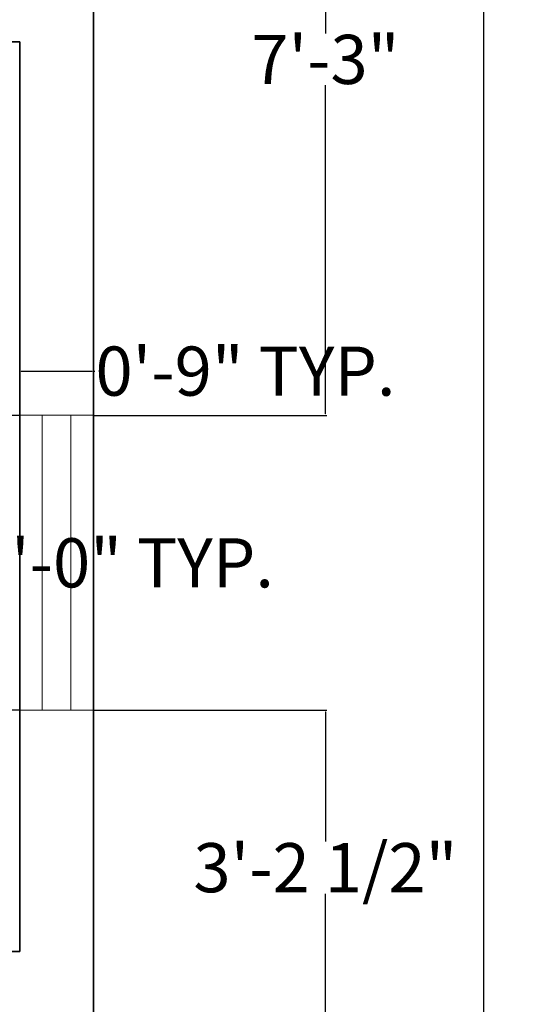
# Model space of a CAD drawing. Units: inches. Extents: x -26 to 575, y -18 to 513.
# Tile 18 of 28: x 513 to 575, y 121 to 241. Entities that reach past the tile are written whole.
import ezdxf

# ---------------------------------------------------------------- set-up
doc = ezdxf.new("R2010")
doc.units = ezdxf.units.IN
doc.header["$MEASUREMENT"] = 0
for name, color, linetype, lineweight in [('A-ANNO-DIMS', 2, 'Continuous', 18), ('A-GLAZ', 4, 'Continuous', 18), ('A-WALL', 7, 'Continuous', 35)]:
    doc.layers.add(name, color=color, linetype=linetype, lineweight=lineweight)
doc.styles.get("Standard").update_dxf_attribs({"font": 'arial.ttf', "height": 6})
doc.dimstyles.get("Standard").update_dxf_attribs({"dimtxt": 6, "dimasz": 0.18, "dimexe": 0.18, "dimexo": 0.0625, "dimgap": 0.09, "dimtad": 0, "dimtih": 1, "dimtoh": 1, "dimzin": 0, "dimdsep": 46, "dimlunit": 3, "dimtxsty": 'Standard', "dimcen": 0.09, "dimadec": 0, "dimazin": 0, "dimtfac": 1, "dimtofl": 0, "dimtmove": 0, "dimatfit": 3, "dimfxl": 1, "dimtolj": 1, "dimtzin": 0, "dimarcsym": 0})

# ---------------------------------------------------------------- blocks, each defined once
blk = doc.blocks.new('*D2')
at = {"layer": 'A-ANNO-DIMS', "color": 0, "lineweight": -2, "transparency": 16777216}
for p, q in [((522.24, 475.51), (569.98, 475.51)), ((569.8, 475.33), (569.8, 250.66)), ((569.8, 19.69), (569.8, 244.35)), ((522.24, 19.51), (569.98, 19.51))]:
    blk.add_line(p, q, dxfattribs=at)
at = {"layer": 'A-ANNO-DIMS', "color": 0, "transparency": 16777216}
for points in [[(569.77, 475.33), (569.83, 475.33), (569.8, 475.51)], [(569.77, 19.69), (569.83, 19.69), (569.8, 19.51)]]:
    blk.add_solid(points, dxfattribs=at)
at = {"layer": 'Defpoints', "color": 0, "transparency": 16777216}
for p in [(522.18, 475.51), (522.18, 19.51), (569.8, 19.51)]:
    blk.add_point(p, dxfattribs=at)
at = {"layer": 'A-ANNO-DIMS', "color": 0, "transparency": 16777216, "insert": (569.8, 247.51), "char_height": 6, "attachment_point": 5}
blk.add_mtext("\\A1;38'", dxfattribs=at)
blk = doc.blocks.new('WINDOW-36IN')
for p, q in [((36, 9), (0, 9)), ((0, 9), (0, 0)), ((36, 0), (36, 9)), ((36, 6.25), (0, 6.25)), ((36, 0), (36, 4.5)), ((36, 2.75), (0, 2.75)), ((0, 0), (36, 0))]:
    blk.add_line(p, q)
blk = doc.blocks.new('*D22')
at = {"layer": 'A-ANNO-DIMS', "color": 0, "lineweight": -2, "transparency": 16777216}
for p, q in [((513.11, 192.93), (507.6, 192.93)), ((507.78, 192.75), (507.78, 178.13)), ((507.78, 157.11), (507.78, 171.74)), ((513.11, 156.93), (507.6, 156.93))]:
    blk.add_line(p, q, dxfattribs=at)
at = {"layer": 'A-ANNO-DIMS', "color": 0, "transparency": 16777216}
for points in [[(507.75, 192.75), (507.81, 192.75), (507.78, 192.93)], [(507.75, 157.11), (507.81, 157.11), (507.78, 156.93)]]:
    blk.add_solid(points, dxfattribs=at)
at = {"layer": 'Defpoints', "color": 0, "transparency": 16777216}
for p in [(507.78, 192.93), (513.18, 192.93), (513.18, 156.93)]:
    blk.add_point(p, dxfattribs=at)
at = {"layer": 'A-ANNO-DIMS', "color": 0, "transparency": 16777216, "insert": (507.78, 174.93), "char_height": 6, "attachment_point": 5}
blk.add_mtext('\\A1;WINDOW 3\'-0" TYP.', dxfattribs=at)
blk = doc.blocks.new('*D23')
at = {"layer": 'A-ANNO-DIMS', "color": 0, "lineweight": -2, "transparency": 16777216}
for p, q in [((513.18, 193), (513.18, 198.51)), ((513.36, 198.33), (522, 198.33)), ((522.18, 193), (522.18, 198.51)), ((522.18, 198.33), (522.36, 198.33))]:
    blk.add_line(p, q, dxfattribs=at)
at = {"layer": 'A-ANNO-DIMS', "color": 0, "transparency": 16777216}
for points in [[(513.36, 198.36), (513.36, 198.3), (513.18, 198.33)], [(522, 198.36), (522, 198.3), (522.18, 198.33)]]:
    blk.add_solid(points, dxfattribs=at)
at = {"layer": 'Defpoints', "color": 0, "transparency": 16777216}
for p in [(522.18, 198.33), (513.18, 192.93), (522.18, 192.93)]:
    blk.add_point(p, dxfattribs=at)
at = {"layer": 'A-ANNO-DIMS', "color": 0, "transparency": 16777216, "insert": (540.73, 198.33), "char_height": 6, "attachment_point": 5}
blk.add_mtext('\\A1;0\'-9" TYP.', dxfattribs=at)
blk = doc.blocks.new('*D42')
at = {"layer": 'A-ANNO-DIMS', "color": 0, "lineweight": -2, "transparency": 16777216}
for p, q in [((522.24, 156.93), (550.66, 156.93)), ((550.48, 156.75), (550.48, 140.92)), ((550.48, 118.69), (550.48, 134.53)), ((522.24, 118.51), (550.66, 118.51))]:
    blk.add_line(p, q, dxfattribs=at)
at = {"layer": 'A-ANNO-DIMS', "color": 0, "transparency": 16777216}
for points in [[(550.45, 156.75), (550.51, 156.75), (550.48, 156.93)], [(550.45, 118.69), (550.51, 118.69), (550.48, 118.51)]]:
    blk.add_solid(points, dxfattribs=at)
at = {"layer": 'Defpoints', "color": 0, "transparency": 16777216}
for p in [(522.18, 156.93), (522.18, 118.51), (550.48, 118.51)]:
    blk.add_point(p, dxfattribs=at)
at = {"layer": 'A-ANNO-DIMS', "color": 0, "transparency": 16777216, "insert": (550.48, 137.72), "char_height": 6, "attachment_point": 5}
blk.add_mtext('\\A1;3\'-2 1/2"', dxfattribs=at)
blk = doc.blocks.new('*D43')
at = {"layer": 'A-ANNO-DIMS', "color": 0, "lineweight": -2, "transparency": 16777216}
for p, q in [((522.24, 279.8), (550.66, 279.8)), ((550.48, 279.62), (550.48, 239.53)), ((550.48, 193.11), (550.48, 233.21)), ((522.24, 192.93), (550.66, 192.93))]:
    blk.add_line(p, q, dxfattribs=at)
at = {"layer": 'A-ANNO-DIMS', "color": 0, "transparency": 16777216}
for points in [[(550.45, 279.62), (550.51, 279.62), (550.48, 279.8)], [(550.45, 193.11), (550.51, 193.11), (550.48, 192.93)]]:
    blk.add_solid(points, dxfattribs=at)
at = {"layer": 'Defpoints', "color": 0, "transparency": 16777216}
for p in [(522.18, 279.8), (550.48, 279.8), (522.18, 192.93)]:
    blk.add_point(p, dxfattribs=at)
at = {"layer": 'A-ANNO-DIMS', "color": 0, "transparency": 16777216, "insert": (550.48, 236.37), "char_height": 6, "attachment_point": 5}
blk.add_mtext('\\A1;7\'-3"', dxfattribs=at)

msp = doc.modelspace()

# ---------------------------------------------------------------- linework, layer by layer
at = {"layer": 'A-WALL'}
for p, q in [((513.177, 238.508), (378.677, 238.508)), ((513.177, 127.508), (513.177, 238.508)), ((513.177, 127.508), (378.677, 127.508))]:
    msp.add_line(p, q, dxfattribs=at)
msp.add_lwpolyline([(18.177, 19.508), (522.177, 19.508), (522.177, 475.508), (18.177, 475.508)], close=True, dxfattribs=at)

# ---------------------------------------------------------------- block references
at = {"layer": 'A-GLAZ', "extrusion": (0, 0, -1), "zscale": -1, "rotation": 90}
msp.add_blockref('WINDOW-36IN', (-513.177, 156.935), dxfattribs=at)

# ---------------------------------------------------------------- dimensions: what is measured, and where the dimension line sits
at = {"layer": 'A-ANNO-DIMS'}
for base, p1, p2, override, picture, middle in [((569.801, 19.508), (522.177, 475.508), (522.177, 19.508), {"dimclrd": 0, "dimclre": 0, "dimclrt": 0}, '*D2', (569.801, 247.508)), ((550.477, 279.805), (522.177, 192.934), (522.177, 279.805), {"dimdec": 1, "dimlfac": 1, "dimrnd": 0, "dimzin": 1, "dimdsep": 46, "dimlunit": 4, "dimfrac": 2}, '*D43', (550.477, 236.37)), ((550.477, 118.508), (522.177, 156.934), (522.177, 118.508), {"dimdec": 1, "dimlfac": 1, "dimrnd": 0, "dimzin": 1, "dimdsep": 46, "dimlunit": 4, "dimfrac": 2}, '*D42', (550.477, 137.721))]:
    dim = msp.add_linear_dim(base=base, p1=p1, p2=p2, angle=90, dimstyle='Standard', override=override, dxfattribs=at)
    dim.commit()
    dim.dimension.update_dxf_attribs({"geometry": picture, "text_midpoint": middle})
dim = msp.add_linear_dim(base=(522.177, 198.334), p1=(513.177, 192.934), p2=(522.177, 192.934), text='<> TYP.', dimstyle='Standard', override={"dimdec": 1, "dimlfac": 1, "dimrnd": 0, "dimzin": 1, "dimdsep": 46, "dimlunit": 4, "dimfrac": 2}, dxfattribs=at)
dim.commit()
dim.dimension.update_dxf_attribs({"geometry": '*D23', "text_midpoint": (540.734, 198.334)})
dim = msp.add_linear_dim(base=(507.777, 192.934), p1=(513.177, 156.934), p2=(513.177, 192.934), angle=90, text='WINDOW <> TYP.', dimstyle='Standard', override={"dimdec": 1, "dimlfac": 1, "dimrnd": 0, "dimzin": 1, "dimdsep": 46, "dimlunit": 4, "dimfrac": 2}, dxfattribs=at)
dim.commit()
dim.dimension.update_dxf_attribs({"geometry": '*D22', "text_midpoint": (507.777, 174.934)})

doc.saveas('drawing.dxf')
